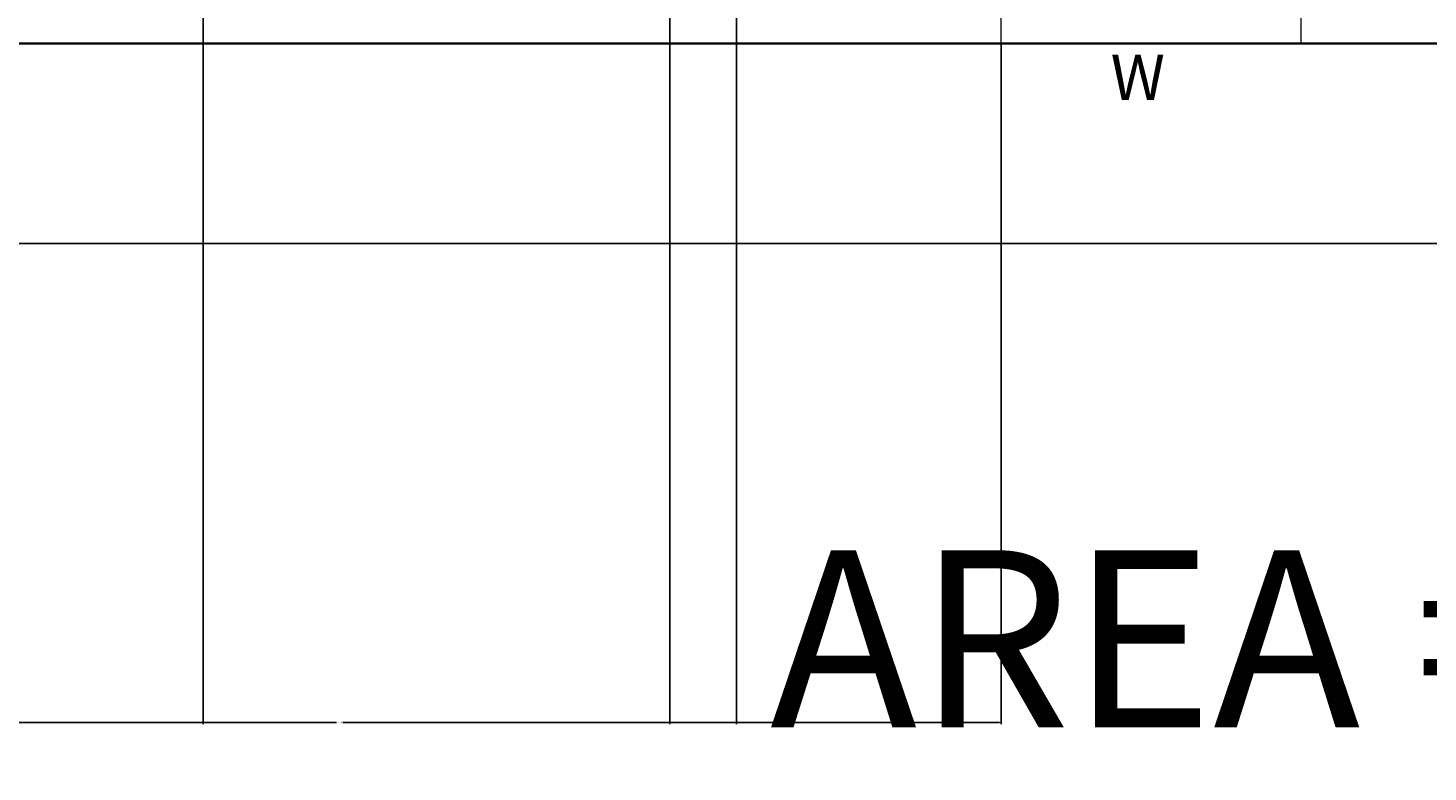
# Model space of a CAD drawing. Units: inches. Extents: x 318 to 927, y -1130 to 13.
# Tile 2 of 17: x 431 to 599, y -1130 to -1041. Entities that reach past the tile are written whole.
import ezdxf

# ---------------------------------------------------------------- set-up
doc = ezdxf.new("R2010")
doc.units = ezdxf.units.IN
doc.header["$MEASUREMENT"] = 0
for name, color, linetype, lineweight in [('A-ANNO-DIMS', 1, 'Continuous', 18), ('A-ANNO-IDEN', 1, 'Continuous', 13), ('A-ANNO-TEXT', 8, 'Continuous', 25), ('wall', 1, 'Continuous', 35), ('win', 5, 'Continuous', 18)]:
    doc.layers.add(name, color=color, linetype=linetype, lineweight=lineweight)
doc.styles.get("Standard").update_dxf_attribs({"font": 'arial.ttf'})
doc.dimstyles.get("Standard").update_dxf_attribs({"dimtxt": 0.18, "dimasz": 0.18, "dimexe": 0.18, "dimexo": 0.0625, "dimgap": 0.09, "dimtad": 0, "dimtih": 1, "dimtoh": 1, "dimdec": 1, "dimzin": 0, "dimdsep": 46, "dimlunit": 4, "dimtxsty": 'Standard', "dimcen": 0.09, "dimadec": 0, "dimazin": 0, "dimtfac": 1, "dimtdec": 1, "dimtofl": 0, "dimtmove": 0, "dimatfit": 3, "dimfxl": 1, "dimtolj": 1, "dimtzin": 0, "dimarcsym": 0})

# ---------------------------------------------------------------- blocks, each defined once
blk = doc.blocks.new('WIN-36IN')
for p, q in [((0, 36), (9, 36)), ((3.5, 36), (3.5, 0)), ((5.5, 36), (5.5, 0)), ((0, 0), (9, 0))]:
    blk.add_line(p, q)
blk = doc.blocks.new('*D26')
at = {"layer": 'A-ANNO-DIMS', "color": 0, "lineweight": -2, "transparency": 16777216}
for p, q in [((645.89, -1042.91), (331.21, -1042.91)), ((331.39, -1043.09), (331.39, -1054.73)), ((331.39, -1066.73), (331.39, -1055.09)), ((645.89, -1066.91), (331.21, -1066.91))]:
    blk.add_line(p, q, dxfattribs=at)
at = {"layer": 'A-ANNO-DIMS', "color": 0, "transparency": 16777216}
for points in [[(331.36, -1043.09), (331.42, -1043.09), (331.39, -1042.91)], [(331.36, -1066.73), (331.42, -1066.73), (331.39, -1066.91)]]:
    blk.add_solid(points, dxfattribs=at)
at = {"layer": 'Defpoints', "color": 0, "transparency": 16777216}
for p in [(645.95, -1042.91), (331.39, -1066.91), (645.95, -1066.91)]:
    blk.add_point(p, dxfattribs=at)
at = {"layer": 'A-ANNO-DIMS', "color": 0, "transparency": 16777216, "insert": (331.39, -1054.91), "char_height": 0.18, "attachment_point": 5}
blk.add_mtext('\\A1;2\'-0"', dxfattribs=at)
blk = doc.blocks.new('*D35')
at = {"layer": 'A-ANNO-DIMS', "color": 0, "lineweight": -2, "transparency": 16777216}
for p, q in [((397.89, -457.98), (397.89, -1124.59)), ((451.89, -457.98), (451.89, -1124.59)), ((398.07, -1124.41), (424.56, -1124.41)), ((451.71, -1124.41), (425.23, -1124.41))]:
    blk.add_line(p, q, dxfattribs=at)
at = {"layer": 'A-ANNO-DIMS', "color": 0, "transparency": 16777216}
for points in [[(398.07, -1124.38), (398.07, -1124.44), (397.89, -1124.41)], [(451.71, -1124.38), (451.71, -1124.44), (451.89, -1124.41)]]:
    blk.add_solid(points, dxfattribs=at)
at = {"layer": 'Defpoints', "color": 0, "transparency": 16777216}
for p in [(397.89, -457.91), (451.89, -457.91), (451.89, -1124.41)]:
    blk.add_point(p, dxfattribs=at)
at = {"layer": 'A-ANNO-DIMS', "color": 0, "transparency": 16777216, "insert": (424.89, -1124.41), "char_height": 0.18, "attachment_point": 5}
blk.add_mtext('\\A1;4\'-6"', dxfattribs=at)
blk = doc.blocks.new('*D36')
at = {"layer": 'A-ANNO-DIMS', "color": 0, "lineweight": -2, "transparency": 16777216}
for p, q in [((507.89, -457.98), (507.89, -1124.59)), ((515.89, -457.98), (515.89, -1124.59)), ((508.07, -1124.41), (511.57, -1124.41)), ((515.71, -1124.41), (512.22, -1124.41))]:
    blk.add_line(p, q, dxfattribs=at)
at = {"layer": 'A-ANNO-DIMS', "color": 0, "transparency": 16777216}
for points in [[(508.07, -1124.38), (508.07, -1124.44), (507.89, -1124.41)], [(515.71, -1124.38), (515.71, -1124.44), (515.89, -1124.41)]]:
    blk.add_solid(points, dxfattribs=at)
at = {"layer": 'Defpoints', "color": 0, "transparency": 16777216}
for p in [(507.89, -457.91), (515.89, -457.91), (515.89, -1124.41)]:
    blk.add_point(p, dxfattribs=at)
at = {"layer": 'A-ANNO-DIMS', "color": 0, "transparency": 16777216, "insert": (511.89, -1124.41), "char_height": 0.18, "attachment_point": 5}
blk.add_mtext('\\A1;0\'-8"', dxfattribs=at)
blk = doc.blocks.new('*D71')
at = {"layer": 'A-ANNO-DIMS', "color": 0, "lineweight": -2, "transparency": 16777216}
for p, q in [((388.89, -1042.98), (388.89, -1124.59)), ((547.67, -1042.98), (547.67, -1124.59)), ((389.07, -1124.41), (467.89, -1124.41)), ((547.49, -1124.41), (468.67, -1124.41))]:
    blk.add_line(p, q, dxfattribs=at)
at = {"layer": 'A-ANNO-DIMS', "color": 0, "transparency": 16777216}
for points in [[(389.07, -1124.38), (389.07, -1124.44), (388.89, -1124.41)], [(547.49, -1124.38), (547.49, -1124.44), (547.67, -1124.41)]]:
    blk.add_solid(points, dxfattribs=at)
at = {"layer": 'Defpoints', "color": 0, "transparency": 16777216}
for p in [(388.89, -1042.91), (547.67, -1042.91), (547.67, -1124.41)]:
    blk.add_point(p, dxfattribs=at)
at = {"layer": 'A-ANNO-DIMS', "color": 0, "transparency": 16777216, "insert": (468.28, -1124.41), "char_height": 0.18, "attachment_point": 5}
blk.add_mtext('\\A1;13\'-3"', dxfattribs=at)

msp = doc.modelspace()

# ---------------------------------------------------------------- linework, layer by layer
at = {"layer": 'wall'}
msp.add_line((388.89, -1042.91), (650.89, -1042.91), dxfattribs=at)

# ---------------------------------------------------------------- block references
at = {"layer": 'win', "rotation": 89.99999999999967}
msp.add_blockref('WIN-36IN', (583.67, -1042.91), dxfattribs=at)

# ---------------------------------------------------------------- texts
at = {"layer": 'A-ANNO-IDEN'}
msp.add_text('W', height=5.44, dxfattribs=at).set_placement((560.81, -1049.69))
at = {"layer": 'A-ANNO-TEXT', "insert": (519.93, -1103.71), "char_height": 21.2807, "attachment_point": 1}
msp.add_mtext_dynamic_manual_height_columns('AREA = 3200 SQFT', width=291.6706, gutter_width=3.55, heights=[0], dxfattribs=at)

# ---------------------------------------------------------------- dimensions: what is measured, and where the dimension line sits
at = {"layer": 'A-ANNO-DIMS'}
for base, p1, p2, picture, middle in [((451.89, -1124.41), (397.89, -457.91), (451.89, -457.91), '*D35', (424.89, -1124.41)), ((515.89, -1124.41), (507.89, -457.91), (515.89, -457.91), '*D36', (511.89, -1124.41)), ((547.67, -1124.41), (388.89, -1042.91), (547.67, -1042.91), '*D71', (468.28, -1124.41))]:
    dim = msp.add_linear_dim(base=base, p1=p1, p2=p2, dimstyle='Standard', override={"dimdec": 1, "dimlfac": 1, "dimrnd": 0, "dimzin": 1, "dimdsep": 46, "dimlunit": 4, "dimfrac": 2}, dxfattribs=at)
    dim.commit()
    dim.dimension.update_dxf_attribs({"geometry": picture, "text_midpoint": middle})
dim = msp.add_linear_dim(base=(331.39, -1066.91), p1=(645.95, -1042.91), p2=(645.95, -1066.91), angle=90, dimstyle='Standard', override={"dimdec": 1, "dimlfac": 1, "dimrnd": 0, "dimzin": 1, "dimdsep": 46, "dimlunit": 4, "dimfrac": 2}, dxfattribs=at)
dim.commit()
dim.dimension.update_dxf_attribs({"geometry": '*D26', "text_midpoint": (331.39, -1054.91)})

doc.saveas('drawing.dxf')
